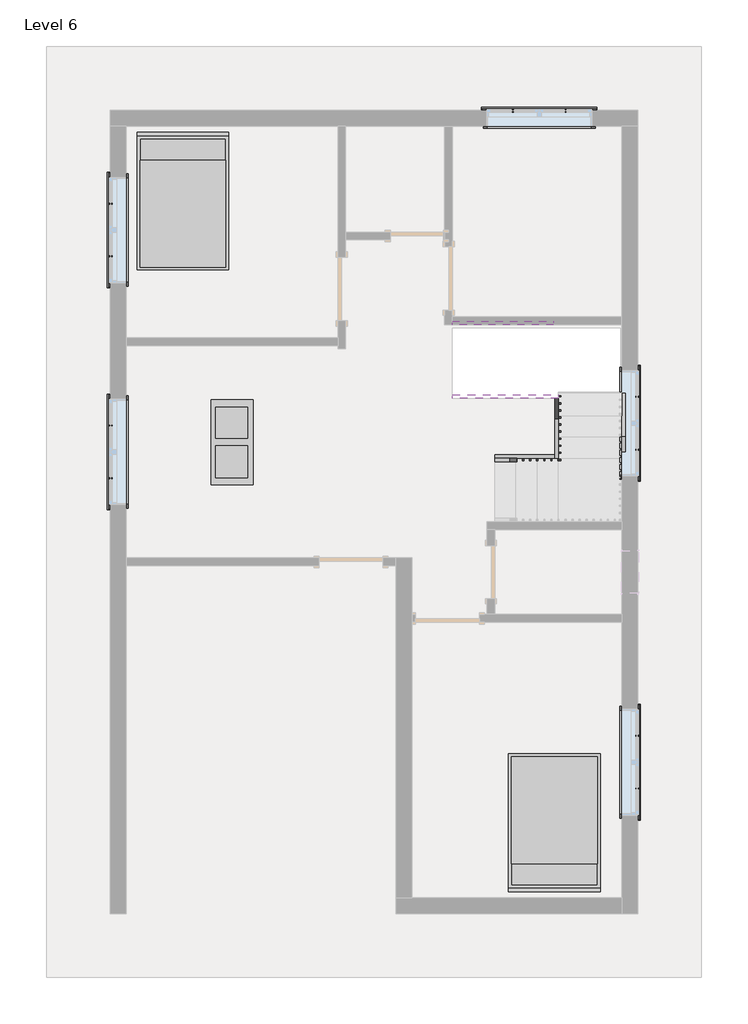
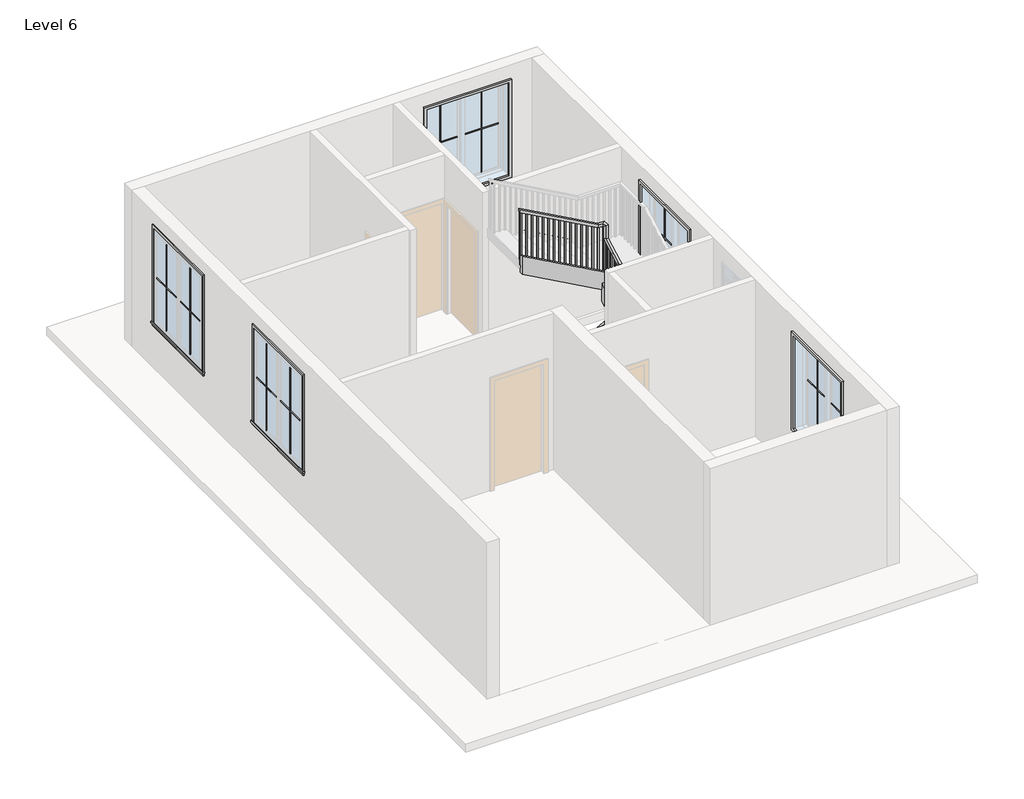
# One storey, part 2 of 2: 21 proxies, 6 members, 2 furniture elements, 1 railing.
"""IFC4 building model written with IfcOpenShell, lengths in millimetres."""

from ifc_helpers import new_model, si_unit, frame, origin, place, context, project, spatial, polyline, outline, extrude, faceted_brep, transform, mapped, element, save
from components import muntin_pattern_2x2_muntin_pattern_2x2_f6a80940, muntin_pattern_2x2_muntin_pattern_2x2_09b00a1c, trim_window_exterior_flat_with_sill_698ed857, trim_window_interior_flat_picture_frame_92551a5e, coffee_table_with_brass_mullions_11320_coffee_table_with_5962bef7, bed_17739_bed_17739_15c61121

model = new_model("IFC4")

# Units and contexts
model_context = context("Model", 3, world=origin())
ifc_project = project(units=[si_unit("LENGTHUNIT", "METRE", prefix="MILLI")], contexts=[model_context])

# Site, building, storey
site = spatial("IfcSite", under=ifc_project)
building = spatial("IfcBuilding", under=site)
storey = spatial("IfcBuildingStorey", under=building, Name="Level 6", Elevation=12801.6)

# Proxies
placement = place(None, origin())
muntin_pattern_2x2_muntin_pattern_2x2_shape = muntin_pattern_2x2_muntin_pattern_2x2_f6a80940(model_context)
element("IfcBuildingElementProxy", 1, Name="Muntin Pattern_2x2 : Muntin Pattern_2x2", ObjectType="Muntin Pattern_2x2 : Muntin Pattern_2x2", at=placement, inside=storey, context=model_context, shape_type="MappedRepresentation", body=[
    mapped(muntin_pattern_2x2_muntin_pattern_2x2_shape, transform((-4589.1575206, 441.8004493, 13785.85), x_axis=(0.0, 1.0, 0.0), y_axis=(-1.0, 0.0, 0.0), z_axis=(0.0, 0.0, 1.0))),
])
element("IfcBuildingElementProxy", 2, Name="Muntin Pattern_2x2 : Muntin Pattern_2x2", ObjectType="Muntin Pattern_2x2 : Muntin Pattern_2x2", at=placement, inside=storey, context=model_context, shape_type="MappedRepresentation", body=[
    mapped(muntin_pattern_2x2_muntin_pattern_2x2_shape, transform((-4589.1575206, 3632.6754493, 13785.85), x_axis=(0.0, 1.0, 0.0), y_axis=(-1.0, 0.0, 0.0), z_axis=(0.0, 0.0, 1.0))),
])
element("IfcBuildingElementProxy", 3, Name="Muntin Pattern_2x2 : Muntin Pattern_2x2", ObjectType="Muntin Pattern_2x2 : Muntin Pattern_2x2", at=placement, inside=storey, context=model_context, shape_type="MappedRepresentation", body=[
    mapped(muntin_pattern_2x2_muntin_pattern_2x2_shape, transform((1197.2799794, 5726.5879493, 13785.85), x_axis=(1.0, 0.0, 0.0), y_axis=(0.0, 1.0, 0.0), z_axis=(0.0, 0.0, 1.0))),
])
element("IfcBuildingElementProxy", 4, Name="Muntin Pattern_2x2 : Muntin Pattern_2x2", ObjectType="Muntin Pattern_2x2 : Muntin Pattern_2x2", at=placement, inside=storey, context=model_context, shape_type="MappedRepresentation", body=[
    mapped(muntin_pattern_2x2_muntin_pattern_2x2_shape, transform((2986.3924794, 1613.3754493, 13785.85), x_axis=(0.0, -1.0, 0.0), y_axis=(1.0, 0.0, 0.0), z_axis=(0.0, 0.0, 1.0))),
])
element("IfcBuildingElementProxy", 5, Name="Muntin Pattern_2x2 : Muntin Pattern_2x2", ObjectType="Muntin Pattern_2x2 : Muntin Pattern_2x2", at=placement, inside=storey, context=model_context, shape_type="MappedRepresentation", body=[
    mapped(muntin_pattern_2x2_muntin_pattern_2x2_shape, transform((2986.3924794, -3260.2495507, 13785.85), x_axis=(0.0, -1.0, 0.0), y_axis=(1.0, 0.0, 0.0), z_axis=(0.0, 0.0, 1.0))),
])
muntin_pattern_2x2_muntin_pattern_2x2_2_shape = muntin_pattern_2x2_muntin_pattern_2x2_09b00a1c(model_context)
element("IfcBuildingElementProxy", 6, Name="Muntin Pattern_2x2 : Muntin Pattern_2x2", ObjectType="Muntin Pattern_2x2 : Muntin Pattern_2x2", at=placement, inside=storey, context=model_context, shape_type="MappedRepresentation", body=[
    mapped(muntin_pattern_2x2_muntin_pattern_2x2_2_shape, transform((-4589.1575206, 1200.6254493, 13785.85), x_axis=(0.0, -1.0, 0.0), y_axis=(1.0, 0.0, 0.0), z_axis=(0.0, 0.0, 1.0))),
])
element("IfcBuildingElementProxy", 7, Name="Muntin Pattern_2x2 : Muntin Pattern_2x2", ObjectType="Muntin Pattern_2x2 : Muntin Pattern_2x2", at=placement, inside=storey, context=model_context, shape_type="MappedRepresentation", body=[
    mapped(muntin_pattern_2x2_muntin_pattern_2x2_2_shape, transform((-4589.1575206, 4391.5004493, 13785.85), x_axis=(0.0, -1.0, 0.0), y_axis=(1.0, 0.0, 0.0), z_axis=(0.0, 0.0, 1.0))),
])
element("IfcBuildingElementProxy", 8, Name="Muntin Pattern_2x2 : Muntin Pattern_2x2", ObjectType="Muntin Pattern_2x2 : Muntin Pattern_2x2", at=placement, inside=storey, context=model_context, shape_type="MappedRepresentation", body=[
    mapped(muntin_pattern_2x2_muntin_pattern_2x2_2_shape, transform((1956.1049794, 5726.5879493, 13785.85), x_axis=(-1.0, 0.0, 0.0), y_axis=(0.0, -1.0, 0.0), z_axis=(0.0, 0.0, 1.0))),
])
element("IfcBuildingElementProxy", 9, Name="Muntin Pattern_2x2 : Muntin Pattern_2x2", ObjectType="Muntin Pattern_2x2 : Muntin Pattern_2x2", at=placement, inside=storey, context=model_context, shape_type="MappedRepresentation", body=[
    mapped(muntin_pattern_2x2_muntin_pattern_2x2_2_shape, transform((2986.3924794, 854.5504493, 13785.85), x_axis=(0.0, 1.0, 0.0), y_axis=(-1.0, 0.0, 0.0), z_axis=(0.0, 0.0, 1.0))),
])
element("IfcBuildingElementProxy", 10, Name="Muntin Pattern_2x2 : Muntin Pattern_2x2", ObjectType="Muntin Pattern_2x2 : Muntin Pattern_2x2", at=placement, inside=storey, context=model_context, shape_type="MappedRepresentation", body=[
    mapped(muntin_pattern_2x2_muntin_pattern_2x2_2_shape, transform((2986.3924794, -4019.0745507, 13785.85), x_axis=(0.0, 1.0, 0.0), y_axis=(-1.0, 0.0, 0.0), z_axis=(0.0, 0.0, 1.0))),
])
trim_window_exterior_flat_with_sill_shape = trim_window_exterior_flat_with_sill_698ed857(model_context)
element("IfcBuildingElementProxy", 11, Name="Trim-Window-Exterior-Flat : with Sill", ObjectType="Trim-Window-Exterior-Flat : with Sill", at=placement, inside=storey, context=model_context, shape_type="MappedRepresentation", body=[
    mapped(trim_window_exterior_flat_with_sill_shape, transform((-4598.6825206, 821.2129493, 15544.8), x_axis=(0.0, -1.0, 0.0), y_axis=(0.0, 0.0, 1.0), z_axis=(-1.0, 0.0, 0.0))),
])
element("IfcBuildingElementProxy", 12, Name="Trim-Window-Exterior-Flat : with Sill", ObjectType="Trim-Window-Exterior-Flat : with Sill", at=placement, inside=storey, context=model_context, shape_type="MappedRepresentation", body=[
    mapped(trim_window_exterior_flat_with_sill_shape, transform((-4598.6825206, 4012.0879493, 15544.8), x_axis=(0.0, -1.0, 0.0), y_axis=(0.0, 0.0, 1.0), z_axis=(-1.0, 0.0, 0.0))),
])
element("IfcBuildingElementProxy", 13, Name="Trim-Window-Exterior-Flat : with Sill", ObjectType="Trim-Window-Exterior-Flat : with Sill", at=placement, inside=storey, context=model_context, shape_type="MappedRepresentation", body=[
    mapped(trim_window_exterior_flat_with_sill_shape, transform((1576.6924794, 5736.1129493, 15544.8), x_axis=(-1.0, 0.0, 0.0), y_axis=(0.0, 0.0, 1.0), z_axis=(0.0, 1.0, 0.0))),
])
element("IfcBuildingElementProxy", 14, Name="Trim-Window-Exterior-Flat : with Sill", ObjectType="Trim-Window-Exterior-Flat : with Sill", at=placement, inside=storey, context=model_context, shape_type="MappedRepresentation", body=[
    mapped(trim_window_exterior_flat_with_sill_shape, transform((2995.9174794, 1233.9629493, 15544.8), x_axis=(0.0, 1.0, 0.0), y_axis=(0.0, 0.0, 1.0), z_axis=(1.0, 0.0, 0.0))),
])
element("IfcBuildingElementProxy", 15, Name="Trim-Window-Exterior-Flat : with Sill", ObjectType="Trim-Window-Exterior-Flat : with Sill", at=placement, inside=storey, context=model_context, shape_type="MappedRepresentation", body=[
    mapped(trim_window_exterior_flat_with_sill_shape, transform((2995.9174794, -3639.6620507, 15544.8), x_axis=(0.0, 1.0, 0.0), y_axis=(0.0, 0.0, 1.0), z_axis=(1.0, 0.0, 0.0))),
])
trim_window_interior_flat_picture_frame_shape = trim_window_interior_flat_picture_frame_92551a5e(model_context)
element("IfcBuildingElementProxy", 16, Name="Trim-Window-Interior-Flat : Picture Frame", ObjectType="Trim-Window-Interior-Flat : Picture Frame", at=placement, inside=storey, context=model_context, shape_type="MappedRepresentation", body=[
    mapped(trim_window_interior_flat_picture_frame_shape, transform((-4370.0825206, 821.2129493, 15544.8), x_axis=(0.0, 1.0, 0.0), y_axis=(0.0, 0.0, 1.0), z_axis=(1.0, 0.0, 0.0))),
])
element("IfcBuildingElementProxy", 17, Name="Trim-Window-Interior-Flat : Picture Frame", ObjectType="Trim-Window-Interior-Flat : Picture Frame", at=placement, inside=storey, context=model_context, shape_type="MappedRepresentation", body=[
    mapped(trim_window_interior_flat_picture_frame_shape, transform((-4370.0825206, 4012.0879493, 15544.8), x_axis=(0.0, 1.0, 0.0), y_axis=(0.0, 0.0, 1.0), z_axis=(1.0, 0.0, 0.0))),
])
element("IfcBuildingElementProxy", 18, Name="Trim-Window-Interior-Flat : Picture Frame", ObjectType="Trim-Window-Interior-Flat : Picture Frame", at=placement, inside=storey, context=model_context, shape_type="MappedRepresentation", body=[
    mapped(trim_window_interior_flat_picture_frame_shape, transform((1576.6924794, 5507.5129493, 15544.8), x_axis=(1.0, 0.0, 0.0), y_axis=(0.0, 0.0, 1.0), z_axis=(0.0, -1.0, 0.0))),
])
element("IfcBuildingElementProxy", 19, Name="Trim-Window-Interior-Flat : Picture Frame", ObjectType="Trim-Window-Interior-Flat : Picture Frame", at=placement, inside=storey, context=model_context, shape_type="MappedRepresentation", body=[
    mapped(trim_window_interior_flat_picture_frame_shape, transform((2767.3174794, 1233.9629493, 15544.8), x_axis=(0.0, -1.0, 0.0), y_axis=(0.0, 0.0, 1.0), z_axis=(-1.0, 0.0, 0.0))),
])
element("IfcBuildingElementProxy", 20, Name="Trim-Window-Interior-Flat : Picture Frame", ObjectType="Trim-Window-Interior-Flat : Picture Frame", at=placement, inside=storey, context=model_context, shape_type="MappedRepresentation", body=[
    mapped(trim_window_interior_flat_picture_frame_shape, transform((2767.3174794, -3639.6620507, 15544.8), x_axis=(0.0, -1.0, 0.0), y_axis=(0.0, 0.0, 1.0), z_axis=(-1.0, 0.0, 0.0))),
])
coffee_table_with_brass_mullions_11320_coffee_table_with_shape = coffee_table_with_brass_mullions_11320_coffee_table_with_5962bef7(model_context)
element("IfcBuildingElementProxy", 21, Name="coffee_table_with_brass_mullions_11320 : coffee_table_with_brass_mullions_11320", ObjectType="coffee_table_with_brass_mullions_11320 : coffee_table_with_brass_mullions_11320", at=placement, inside=storey, context=model_context, shape_type="MappedRepresentation", body=[
    mapped(coffee_table_with_brass_mullions_11320_coffee_table_with_shape, transform((-2412.0418112, 1596.9678033, 12801.6), x_axis=(0.0, 1.0, 0.0), y_axis=(-1.0, 0.0, 0.0), z_axis=(0.0, 0.0, 1.0))),
])

# Furniture
bed_17739_bed_17739_shape = bed_17739_bed_17739_15c61121(model_context)
element("IfcFurniture", 22, ObjectType="Bed_17739 : Bed_17739", at=placement, inside=storey, context=model_context, shape_type="MappedRepresentation", body=[
    mapped(bed_17739_bed_17739_shape, transform((-3550.9325206, 4402.6129493, 12801.6), x_axis=(1.0, 0.0, 0.0), y_axis=(0.0, 1.0, 0.0), z_axis=(0.0, 0.0, 1.0))),
])
element("IfcFurniture", 23, ObjectType="Bed_17739 : Bed_17739", at=placement, inside=storey, context=model_context, shape_type="MappedRepresentation", body=[
    mapped(bed_17739_bed_17739_shape, transform((1795.7674794, -4487.3870507, 12801.6), x_axis=(-1.0, 0.0, 0.0), y_axis=(0.0, -1.0, 0.0), z_axis=(0.0, 0.0, 1.0))),
])

# Members
element("IfcMember", 24, ObjectType="Stringer - 2\" Width", at=placement, inside=storey, context=model_context, shape_type="SweptSolid", body=[
    extrude(outline(polyline([(13009.1983948, 938.5174794), (12801.6, 938.5174794), (12801.6, 1192.4619822), (13140.2974984, 1802.1174794), (13488.9761726, 1802.1174794), (13009.1983948, 938.5174794)])), frame((0.0, 732.3129493, 0.0), z_axis=(0.0, 1.0, 0.0), x_axis=(0.0, 0.0, 1.0)), (0.0, 0.0, 1.0), 50.8),
])
element("IfcMember", 25, ObjectType="Stringer - 2\" Width", at=placement, inside=storey, context=model_context, shape_type="SweptSolid", body=[
    extrude(outline(polyline([(732.3129493, 13337.853054), (732.3129493, 13686.5317281), (1595.9129493, 14166.3095059), (1595.9129493, 13817.6308318), (732.3129493, 13337.853054)])), frame((1802.1174794, 0.0, 0.0), z_axis=(1.0, 0.0, 0.0), x_axis=(0.0, 1.0, 0.0)), (0.0, 0.0, 1.0), 50.8),
])
element("IfcMember", 26, ObjectType="Stringer - 2\" Width", at=placement, inside=storey, context=model_context, shape_type="SweptSolid", body=[
    extrude(outline(polyline([(14015.1863873, 1852.9174794), (14363.8650614, 1852.9174794), (15210.5317281, 328.9174794), (14861.853054, 328.9174794), (14015.1863873, 1852.9174794)])), frame((0.0, 1595.9129493, 0.0), z_axis=(0.0, 1.0, 0.0), x_axis=(0.0, 0.0, 1.0)), (0.0, 0.0, 1.0), 50.8),
])
element("IfcMember", 27, ObjectType="Stringer - 2\" Width", at=placement, inside=storey, context=model_context, shape_type="SweptSolid", body=[
    extrude(outline(polyline([(13009.1983948, 938.5174794), (12801.6, 938.5174794), (12801.6, 1192.4619822), (13178.5317281, 1870.9390928), (13178.5317281, 1243.3174794), (13009.1983948, 938.5174794)])), frame((0.0, -232.8870507, 0.0), z_axis=(0.0, 1.0, 0.0), x_axis=(0.0, 0.0, 1.0)), (0.0, 0.0, 1.0), 50.8),
])
element("IfcMember", 28, ObjectType="Stringer - 2\" Width", at=placement, inside=storey, context=model_context, shape_type="SweptSolid", body=[
    extrude(outline(polyline([(714.2913359, 13676.5197207), (1037.1129493, 13855.8650614), (1664.7345627, 13855.8650614), (1341.9129493, 13676.5197207), (714.2913359, 13676.5197207)])), frame((2767.3174794, 0.0, 0.0), z_axis=(1.0, 0.0, 0.0), x_axis=(0.0, 1.0, 0.0)), (0.0, 0.0, 1.0), 50.8),
])
element("IfcMember", 29, ObjectType="Stringer - 2\" Width", at=placement, inside=storey, context=model_context, shape_type="SweptSolid", body=[
    extrude(outline(polyline([(14403.2419429, 1782.0390928), (15210.5317281, 328.9174794), (14861.853054, 328.9174794), (14403.2419429, 1154.4174794), (14403.2419429, 1782.0390928)])), frame((0.0, 2650.0129493, 0.0), z_axis=(0.0, 1.0, 0.0), x_axis=(0.0, 0.0, 1.0)), (0.0, 0.0, 1.0), 50.8),
])

# Railing
element("IfcRailing", 30, ObjectType="Handrail - Rectangular", at=placement, inside=storey, context=model_context, shape_type="SolidModel", body=[
    faceted_brep([(938.5174794, 732.3129493, 13885.3333333), (938.5174794, 732.3129493, 13827.220221), (938.5174794, 681.5129493, 13827.220221), (938.5174794, 681.5129493, 13885.3333333), (1776.7174794, 732.3129493, 14351.0), (1827.5174794, 732.3129493, 14321.1091099), (1827.5174794, 681.5129493, 14321.1091099), (1776.7174794, 681.5129493, 14351.0), (1776.7174794, 732.3129493, 14605.0), (1827.5174794, 732.3129493, 14554.2), (1827.5174794, 681.5129493, 14554.2), (1776.7174794, 681.5129493, 14605.0), (1852.9174794, 732.3129493, 14605.0), (1852.9174794, 732.3129493, 14554.2), (1903.7174794, 681.5129493, 14554.2), (1903.7174794, 681.5129493, 14605.0), (1852.9174794, 808.5129493, 14605.0), (1852.9174794, 821.6765516, 14554.2), (1903.7174794, 821.6765516, 14554.2), (1903.7174794, 808.5129493, 14605.0), (1852.9174794, 1570.5129493, 15028.3333333), (1852.9174794, 1621.3129493, 14998.4424432), (1903.7174794, 1621.3129493, 14998.4424432), (1903.7174794, 1570.5129493, 15028.3333333), (1852.9174794, 1570.5129493, 15282.3333333), (1852.9174794, 1621.3129493, 15231.5333333), (1903.7174794, 1621.3129493, 15231.5333333), (1903.7174794, 1570.5129493, 15282.3333333), (1852.9174794, 1646.7129493, 15282.3333333), (1852.9174794, 1646.7129493, 15231.5333333), (1903.7174794, 1697.5129493, 15231.5333333), (1903.7174794, 1697.5129493, 15282.3333333), (1776.7174794, 1646.7129493, 15282.3333333), (1763.5538772, 1646.7129493, 15231.5333333), (1763.5538772, 1697.5129493, 15231.5333333), (1776.7174794, 1697.5129493, 15282.3333333), (328.9174794, 1646.7129493, 16086.6666667), (328.9174794, 1697.5129493, 16086.6666667), (328.9174794, 1697.5129493, 16028.5535543), (328.9174794, 1646.7129493, 16028.5535543)], [[[0, 1, 2, 3]], [[1, 0, 4, 5]], [[2, 1, 5, 6]], [[3, 2, 6, 7]], [[0, 3, 7, 4]], [[5, 4, 8, 9]], [[6, 5, 9, 10]], [[7, 6, 10, 11]], [[4, 7, 11, 8]], [[9, 8, 12, 13]], [[10, 9, 13, 14]], [[11, 10, 14, 15]], [[8, 11, 15, 12]], [[13, 12, 16, 17]], [[14, 13, 17, 18]], [[15, 14, 18, 19]], [[12, 15, 19, 16]], [[17, 16, 20, 21]], [[18, 17, 21, 22]], [[19, 18, 22, 23]], [[16, 19, 23, 20]], [[21, 20, 24, 25]], [[22, 21, 25, 26]], [[23, 22, 26, 27]], [[20, 23, 27, 24]], [[25, 24, 28, 29]], [[26, 25, 29, 30]], [[27, 26, 30, 31]], [[24, 27, 31, 28]], [[29, 28, 32, 33]], [[30, 29, 33, 34]], [[31, 30, 34, 35]], [[28, 31, 35, 32]], [[36, 37, 38, 39]], [[33, 32, 36, 39]], [[34, 33, 39, 38]], [[35, 34, 38, 37]], [[32, 35, 37, 36]]]),
    extrude(outline(polyline([(16019.7341099, 344.7924794), (15002.9333333, 344.7924794), (15002.9333333, 363.8424794), (16009.1507765, 363.8424794), (16019.7341099, 344.7924794)])), frame((0.0, 1662.5879493, 0.0), z_axis=(0.0, 1.0, 0.0), x_axis=(0.0, 0.0, 1.0)), (0.0, 0.0, 1.0), 19.05),
    extrude(outline(polyline([(15963.2896654, 446.3924794), (15002.9333333, 446.3924794), (15002.9333333, 465.4424794), (15952.7063321, 465.4424794), (15963.2896654, 446.3924794)])), frame((0.0, 1662.5879493, 0.0), z_axis=(0.0, 1.0, 0.0), x_axis=(0.0, 0.0, 1.0)), (0.0, 0.0, 1.0), 19.05),
    extrude(outline(polyline([(15906.845221, 547.9924794), (15002.9333333, 547.9924794), (15002.9333333, 567.0424794), (15896.2618876, 567.0424794), (15906.845221, 547.9924794)])), frame((0.0, 1662.5879493, 0.0), z_axis=(0.0, 1.0, 0.0), x_axis=(0.0, 0.0, 1.0)), (0.0, 0.0, 1.0), 19.05),
    extrude(outline(polyline([(15850.4007765, 649.5924794), (14833.6, 649.5924794), (14833.6, 668.6424794), (15839.8174432, 668.6424794), (15850.4007765, 649.5924794)])), frame((0.0, 1662.5879493, 0.0), z_axis=(0.0, 1.0, 0.0), x_axis=(0.0, 0.0, 1.0)), (0.0, 0.0, 1.0), 19.05),
    extrude(outline(polyline([(15793.9563321, 751.1924794), (14833.6, 751.1924794), (14833.6, 770.2424794), (15783.3729988, 770.2424794), (15793.9563321, 751.1924794)])), frame((0.0, 1662.5879493, 0.0), z_axis=(0.0, 1.0, 0.0), x_axis=(0.0, 0.0, 1.0)), (0.0, 0.0, 1.0), 19.05),
    extrude(outline(polyline([(15737.5118876, 852.7924794), (14833.6, 852.7924794), (14833.6, 871.8424794), (15726.9285543, 871.8424794), (15737.5118876, 852.7924794)])), frame((0.0, 1662.5879493, 0.0), z_axis=(0.0, 1.0, 0.0), x_axis=(0.0, 0.0, 1.0)), (0.0, 0.0, 1.0), 19.05),
    extrude(outline(polyline([(15681.0674432, 954.3924794), (14664.2666667, 954.3924794), (14664.2666667, 973.4424794), (15670.4841099, 973.4424794), (15681.0674432, 954.3924794)])), frame((0.0, 1662.5879493, 0.0), z_axis=(0.0, 1.0, 0.0), x_axis=(0.0, 0.0, 1.0)), (0.0, 0.0, 1.0), 19.05),
    extrude(outline(polyline([(15624.6229988, 1055.9924794), (14664.2666667, 1055.9924794), (14664.2666667, 1075.0424794), (15614.0396654, 1075.0424794), (15624.6229988, 1055.9924794)])), frame((0.0, 1662.5879493, 0.0), z_axis=(0.0, 1.0, 0.0), x_axis=(0.0, 0.0, 1.0)), (0.0, 0.0, 1.0), 19.05),
    extrude(outline(polyline([(15568.1785543, 1157.5924794), (14664.2666667, 1157.5924794), (14664.2666667, 1176.6424794), (15557.595221, 1176.6424794), (15568.1785543, 1157.5924794)])), frame((0.0, 1662.5879493, 0.0), z_axis=(0.0, 1.0, 0.0), x_axis=(0.0, 0.0, 1.0)), (0.0, 0.0, 1.0), 19.05),
    extrude(outline(polyline([(15511.7341099, 1259.1924794), (14494.9333333, 1259.1924794), (14494.9333333, 1278.2424794), (15501.1507765, 1278.2424794), (15511.7341099, 1259.1924794)])), frame((0.0, 1662.5879493, 0.0), z_axis=(0.0, 1.0, 0.0), x_axis=(0.0, 0.0, 1.0)), (0.0, 0.0, 1.0), 19.05),
    extrude(outline(polyline([(15455.2896654, 1360.7924794), (14494.9333333, 1360.7924794), (14494.9333333, 1379.8424794), (15444.7063321, 1379.8424794), (15455.2896654, 1360.7924794)])), frame((0.0, 1662.5879493, 0.0), z_axis=(0.0, 1.0, 0.0), x_axis=(0.0, 0.0, 1.0)), (0.0, 0.0, 1.0), 19.05),
    extrude(outline(polyline([(15398.845221, 1462.3924794), (14494.9333333, 1462.3924794), (14494.9333333, 1481.4424794), (15388.2618876, 1481.4424794), (15398.845221, 1462.3924794)])), frame((0.0, 1662.5879493, 0.0), z_axis=(0.0, 1.0, 0.0), x_axis=(0.0, 0.0, 1.0)), (0.0, 0.0, 1.0), 19.05),
    extrude(outline(polyline([(15342.4007765, 1563.9924794), (14325.6, 1563.9924794), (14325.6, 1583.0424794), (15331.8174432, 1583.0424794), (15342.4007765, 1563.9924794)])), frame((0.0, 1662.5879493, 0.0), z_axis=(0.0, 1.0, 0.0), x_axis=(0.0, 0.0, 1.0)), (0.0, 0.0, 1.0), 19.05),
    extrude(outline(polyline([(15285.9563321, 1665.5924794), (14325.6, 1665.5924794), (14325.6, 1684.6424794), (15275.3729988, 1684.6424794), (15285.9563321, 1665.5924794)])), frame((0.0, 1662.5879493, 0.0), z_axis=(0.0, 1.0, 0.0), x_axis=(0.0, 0.0, 1.0)), (0.0, 0.0, 1.0), 19.05),
    extrude(outline(polyline([(15229.5118876, 1767.1924794), (14325.6, 1767.1924794), (14325.6, 1786.2424794), (15218.9285543, 1786.2424794), (15229.5118876, 1767.1924794)])), frame((0.0, 1662.5879493, 0.0), z_axis=(0.0, 1.0, 0.0), x_axis=(0.0, 0.0, 1.0)), (0.0, 0.0, 1.0), 19.05),
    extrude(outline(polyline([(1868.7924794, 1611.7879493), (1868.7924794, 1630.8379493), (1887.8424794, 1630.8379493), (1887.8424794, 1611.7879493), (1868.7924794, 1611.7879493)])), frame((0.0, 0.0, 13986.9333333), z_axis=(0.0, 0.0, 1.0), x_axis=(1.0, 0.0, 0.0)), (0.0, 0.0, 1.0), 1244.6),
    extrude(outline(polyline([(1529.2379493, 14947.2896654), (1529.2379493, 13986.9333333), (1510.1879493, 13986.9333333), (1510.1879493, 14936.7063321), (1529.2379493, 14947.2896654)])), frame((1868.7924794, 0.0, 0.0), z_axis=(1.0, 0.0, 0.0), x_axis=(0.0, 1.0, 0.0)), (0.0, 0.0, 1.0), 19.05),
    extrude(outline(polyline([(1427.6379493, 14890.845221), (1427.6379493, 13986.9333333), (1408.5879493, 13986.9333333), (1408.5879493, 14880.2618876), (1427.6379493, 14890.845221)])), frame((1868.7924794, 0.0, 0.0), z_axis=(1.0, 0.0, 0.0), x_axis=(0.0, 1.0, 0.0)), (0.0, 0.0, 1.0), 19.05),
    extrude(outline(polyline([(1326.0379493, 14834.4007765), (1326.0379493, 13817.6), (1306.9879493, 13817.6), (1306.9879493, 14823.8174432), (1326.0379493, 14834.4007765)])), frame((1868.7924794, 0.0, 0.0), z_axis=(1.0, 0.0, 0.0), x_axis=(0.0, 1.0, 0.0)), (0.0, 0.0, 1.0), 19.05),
    extrude(outline(polyline([(1224.4379493, 14777.9563321), (1224.4379493, 13817.6), (1205.3879493, 13817.6), (1205.3879493, 14767.3729988), (1224.4379493, 14777.9563321)])), frame((1868.7924794, 0.0, 0.0), z_axis=(1.0, 0.0, 0.0), x_axis=(0.0, 1.0, 0.0)), (0.0, 0.0, 1.0), 19.05),
    extrude(outline(polyline([(1122.8379493, 14721.5118876), (1122.8379493, 13817.6), (1103.7879493, 13817.6), (1103.7879493, 14710.9285543), (1122.8379493, 14721.5118876)])), frame((1868.7924794, 0.0, 0.0), z_axis=(1.0, 0.0, 0.0), x_axis=(0.0, 1.0, 0.0)), (0.0, 0.0, 1.0), 19.05),
    extrude(outline(polyline([(1021.2379493, 14665.0674432), (1021.2379493, 13648.2666667), (1002.1879493, 13648.2666667), (1002.1879493, 14654.4841099), (1021.2379493, 14665.0674432)])), frame((1868.7924794, 0.0, 0.0), z_axis=(1.0, 0.0, 0.0), x_axis=(0.0, 1.0, 0.0)), (0.0, 0.0, 1.0), 19.05),
    extrude(outline(polyline([(919.6379493, 14608.6229988), (919.6379493, 13648.2666667), (900.5879493, 13648.2666667), (900.5879493, 14598.0396654), (919.6379493, 14608.6229988)])), frame((1868.7924794, 0.0, 0.0), z_axis=(1.0, 0.0, 0.0), x_axis=(0.0, 1.0, 0.0)), (0.0, 0.0, 1.0), 19.05),
    extrude(outline(polyline([(818.0379493, 14552.1785543), (818.0379493, 13648.2666667), (798.9879493, 13648.2666667), (798.9879493, 14541.595221), (818.0379493, 14552.1785543)])), frame((1868.7924794, 0.0, 0.0), z_axis=(1.0, 0.0, 0.0), x_axis=(0.0, 1.0, 0.0)), (0.0, 0.0, 1.0), 19.05),
    extrude(outline(polyline([(1843.3924794, 716.4379493), (1862.4424794, 716.4379493), (1862.4424794, 697.3879493), (1843.3924794, 697.3879493), (1843.3924794, 716.4379493)])), frame((0.0, 0.0, 13478.9333333), z_axis=(0.0, 0.0, 1.0), x_axis=(1.0, 0.0, 0.0)), (0.0, 0.0, 1.0), 1075.2666667),
    extrude(outline(polyline([(14273.4841099, 1741.7924794), (13309.6, 1741.7924794), (13309.6, 1760.8424794), (14284.0674432, 1760.8424794), (14273.4841099, 1741.7924794)])), frame((0.0, 697.3879493, 0.0), z_axis=(0.0, 1.0, 0.0), x_axis=(0.0, 0.0, 1.0)), (0.0, 0.0, 1.0), 19.05),
    extrude(outline(polyline([(14217.0396654, 1640.1924794), (13309.6, 1640.1924794), (13309.6, 1659.2424794), (14227.6229988, 1659.2424794), (14217.0396654, 1640.1924794)])), frame((0.0, 697.3879493, 0.0), z_axis=(0.0, 1.0, 0.0), x_axis=(0.0, 0.0, 1.0)), (0.0, 0.0, 1.0), 19.05),
    extrude(outline(polyline([(14160.595221, 1538.5924794), (13309.6, 1538.5924794), (13309.6, 1557.6424794), (14171.1785543, 1557.6424794), (14160.595221, 1538.5924794)])), frame((0.0, 697.3879493, 0.0), z_axis=(0.0, 1.0, 0.0), x_axis=(0.0, 0.0, 1.0)), (0.0, 0.0, 1.0), 19.05),
    extrude(outline(polyline([(14104.1507765, 1436.9924794), (13140.2666667, 1436.9924794), (13140.2666667, 1456.0424794), (14114.7341099, 1456.0424794), (14104.1507765, 1436.9924794)])), frame((0.0, 697.3879493, 0.0), z_axis=(0.0, 1.0, 0.0), x_axis=(0.0, 0.0, 1.0)), (0.0, 0.0, 1.0), 19.05),
    extrude(outline(polyline([(14047.7063321, 1335.3924794), (13140.2666667, 1335.3924794), (13140.2666667, 1354.4424794), (14058.2896654, 1354.4424794), (14047.7063321, 1335.3924794)])), frame((0.0, 697.3879493, 0.0), z_axis=(0.0, 1.0, 0.0), x_axis=(0.0, 0.0, 1.0)), (0.0, 0.0, 1.0), 19.05),
    extrude(outline(polyline([(13991.2618876, 1233.7924794), (13140.2666667, 1233.7924794), (13140.2666667, 1252.8424794), (14001.845221, 1252.8424794), (13991.2618876, 1233.7924794)])), frame((0.0, 697.3879493, 0.0), z_axis=(0.0, 1.0, 0.0), x_axis=(0.0, 0.0, 1.0)), (0.0, 0.0, 1.0), 19.05),
    extrude(outline(polyline([(13934.8174432, 1132.1924794), (12970.9333333, 1132.1924794), (12970.9333333, 1151.2424794), (13945.4007765, 1151.2424794), (13934.8174432, 1132.1924794)])), frame((0.0, 697.3879493, 0.0), z_axis=(0.0, 1.0, 0.0), x_axis=(0.0, 0.0, 1.0)), (0.0, 0.0, 1.0), 19.05),
    extrude(outline(polyline([(13878.3729988, 1030.5924794), (12970.9333333, 1030.5924794), (12970.9333333, 1049.6424794), (13888.9563321, 1049.6424794), (13878.3729988, 1030.5924794)])), frame((0.0, 697.3879493, 0.0), z_axis=(0.0, 1.0, 0.0), x_axis=(0.0, 0.0, 1.0)), (0.0, 0.0, 1.0), 19.05),
    extrude(outline(polyline([(1868.7924794, 1662.5879493), (1868.7924794, 1681.6379493), (1887.8424794, 1681.6379493), (1887.8424794, 1662.5879493), (1868.7924794, 1662.5879493)])), frame((0.0, 0.0, 14156.2666667), z_axis=(0.0, 0.0, 1.0), x_axis=(1.0, 0.0, 0.0)), (0.0, 0.0, 1.0), 1075.2666667),
    extrude(outline(polyline([(1868.7924794, 716.4379493), (1887.8424794, 716.4379493), (1887.8424794, 697.3879493), (1868.7924794, 697.3879493), (1868.7924794, 716.4379493)])), frame((0.0, 0.0, 13478.9333333), z_axis=(0.0, 0.0, 1.0), x_axis=(1.0, 0.0, 0.0)), (0.0, 0.0, 1.0), 1075.2666667),
    extrude(outline(polyline([(16028.5535543, 328.9174794), (15002.9333333, 328.9174794), (15002.9333333, 347.9674794), (16017.970221, 347.9674794), (16028.5535543, 328.9174794)])), frame((0.0, 1662.5879493, 0.0), z_axis=(0.0, 1.0, 0.0), x_axis=(0.0, 0.0, 1.0)), (0.0, 0.0, 1.0), 19.05),
    extrude(outline(polyline([(13827.220221, 938.5174794), (12970.9333333, 938.5174794), (12970.9333333, 957.5674794), (13837.8035543, 957.5674794), (13827.220221, 938.5174794)])), frame((0.0, 697.3879493, 0.0), z_axis=(0.0, 1.0, 0.0), x_axis=(0.0, 0.0, 1.0)), (0.0, 0.0, 1.0), 19.05),
])

save(model, "model.ifc")

# Revit data of these elements
# Type "Muntin Pattern_2x2 : Muntin Pattern_2x2"
#   Width [instance default] = 4' - 0"
#   Thickness = 0' - 0 1/2"
#   Height [instance default] = 4' - 0"
#   Distance = 0' - 0 3/4"
#   Interior Material [instance default] = none
#   Exterior Material [instance default] = none
#   Default Elevation = 0
# Type "Trim-Window-Exterior-Flat : with Sill"
#   Trim Width = 0' - 2 1/4"
#   Trim Thickness_Picture Frame = 0' - 1 1/4"
#   Trim Thickness_with Sill = 0' - 0 3/4"
#   Sill Thickness = 0' - 1 1/4"
#   Opening Width [instance default] = 2' - 0"
#   Opening Height [instance default] = 3' - 0"
#   Default Elevation = 4' - 0"
#   Sill = yes
#   Picture Frame = no
#   Trim Material [instance default] = none
# Type "Trim-Window-Interior-Flat : Picture Frame"
#   Trim Thickness_Picture Frame = 0' - 1 1/4"
#   Trim Width = 0' - 2 1/4"
#   Trim Thickness_with Sill = 0' - 0 3/4"
#   Sill Thickness = 0' - 1 1/4"
#   Opening Width [instance default] = 2' - 0"
#   Opening Height [instance default] = 3' - 0"
#   Default Elevation = 4' - 0"
#   Sill = no
#   Picture Frame = yes
#   Trim Material [instance default] = none
# Type "coffee_table_with_brass_mullions_11320 : coffee_table_with_brass_mullions_11320"
#   Default Elevation = 0
# Type "Bed_17739 : Bed_17739"
#   Default Elevation = 0
# Type "Handrail - Rectangular"
#   Assembly Code = "C2010400"
#   built-in parameter 1008612 = 0.0416667 (stored number, unit not read)
#   built-in parameter 1008611 = 0.0416667 (stored number, unit not read)
#   built-in parameter 1008609 = 0.333333 (stored number, unit not read)
#   built-in parameter 1008604 = 0.166667 (stored number, unit not read)
#   built-in parameter 1008603 = 0.166667 (stored number, unit not read)
#   Railing Height = 3' - 0"
#   built-in parameter 1008630 = 2
#   built-in parameter 1008610 = 2
#   built-in parameter 1008618 = Baluster - Square : 3/4"
# Elements 1, 2, 3, 4, 5, 6, 7, 8, 9, 10 (IfcBuildingElementProxy, "Muntin Pattern_2x2 : Muntin Pattern_2x2")
#   Width = 2' - 0 5/8"
#   Height = 5' - 6 1/2"
#   Interior Material = Wood - Stained
#   Exterior Material = Clad - White
#   Phase Created = New Construction
#   Materials on its faces: "Clad - White", "Wood - Stained"
# Elements 11, 12, 13, 14, 15 (IfcBuildingElementProxy, "Trim-Window-Exterior-Flat : with Sill")
#   Opening Width = 5' - 0"
#   Opening Height = 6' - 0"
#   Trim Material = Clad - White
#   Phase Created = New Construction
#   Materials on its faces: "Clad - White"
# Elements 16, 17, 18, 19, 20 (IfcBuildingElementProxy, "Trim-Window-Interior-Flat : Picture Frame")
#   Opening Width = 5' - 0"
#   Opening Height = 6' - 0"
#   Trim Material = Wood - Stained
#   Phase Created = New Construction
#   Materials on its faces: "Wood - Stained"
# Element 21 (IfcBuildingElementProxy, "coffee_table_with_brass_mullions_11320 : coffee_table_with_brass_mullions_11320")
#   Phase Created = New Construction
#   Materials on its faces: "Default Wall", "TABLE", "Glass", "Default"
# Elements 22, 23 (IfcFurniture, "Bed_17739 : Bed_17739")
#   Phase Created = New Construction
#   Materials on its faces: "legs", "sheets", "bed frame", "Blanket"
# Elements 24, 25, 26, 27, 28, 29 (IfcMember, "Stringer - 2\" Width")
#   Phase Created = New Construction
# Element 30 (IfcRailing, "Handrail - Rectangular")
#   Phase Created = New Construction
# Materials
#   "Clad - White": class "Wood", colour RGB 242 242 238, transparency 0, Cost = 0
#   "Wood - Stained": class "Wood", colour RGB 224 178 126, transparency 0, Cost = 0
#   "Default Wall": colour RGB 128 128 128, transparency 0, Cost = 0
#   "TABLE": class "Generic", colour RGB 120 120 120, transparency 0, Cost = 0
#   "Glass": class "Glass", colour RGB 0 128 192, transparency 0.75, Description = "Soda Lime Glass", Cost = 0
#   "Default": colour RGB 127 127 127, transparency 0, Cost = 0
#   "legs": colour RGB 90 73 37, transparency 0, Cost = 0
#   "sheets": colour RGB 200 195 176, transparency 0, Cost = 0
#   "bed frame": colour RGB 90 73 37, transparency 0, Cost = 0
#   "Blanket": class "System", colour RGB 59 0 1, transparency 0, Cost = 0
